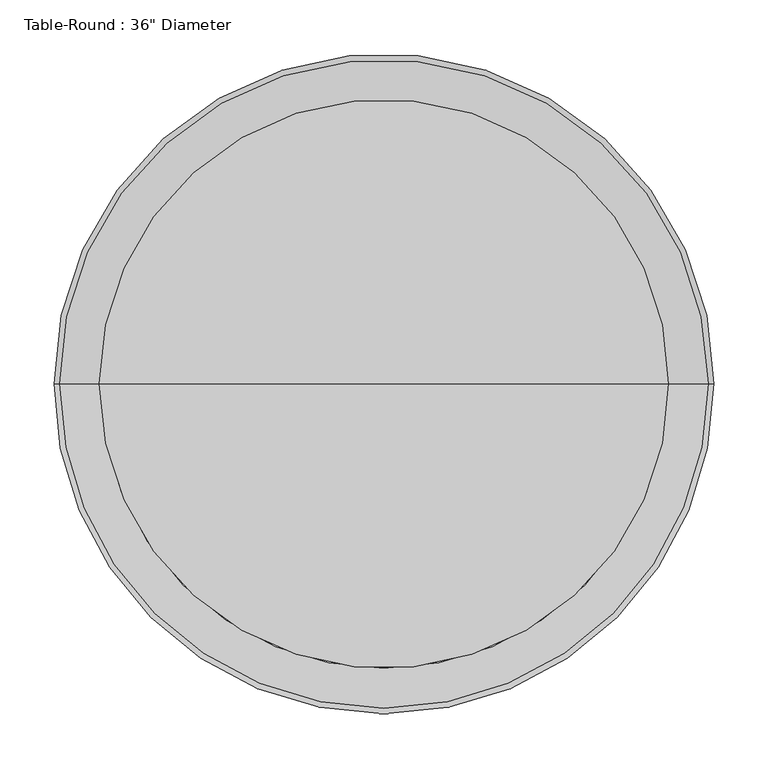
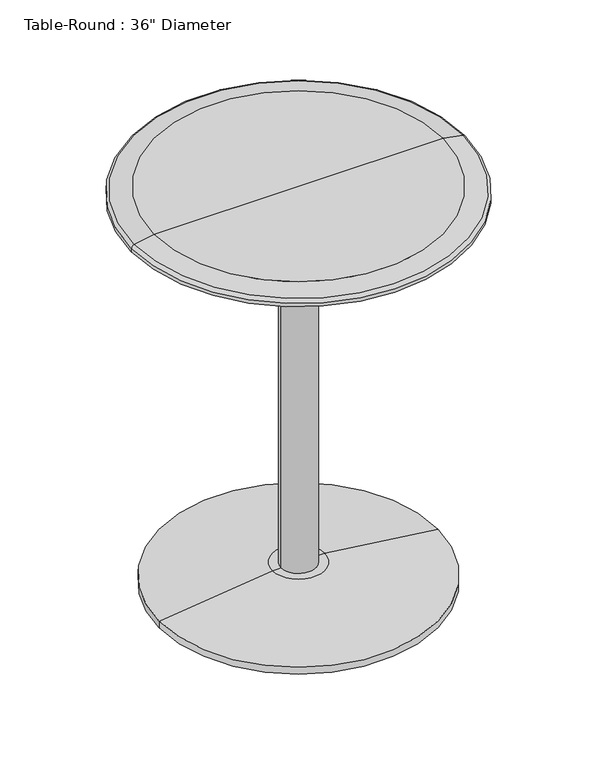
"""IFC4 building model written with IfcOpenShell, lengths in millimetres: furniture geometry."""

from ifc_helpers import new_model, si_unit, point, frame, origin, origin_2d, place, context, project, spatial, polyline, circle_curve, ellipse_curve, trimmed, segment, composite_curve, outline, extrude, source, transform, mapped, element, save
from ifc_brep_helpers import plane_surface, cylinder_surface, revolved_surface, advanced_brep


def furniture_a0cc3393(model_context):
    return source(origin(), model_context, "Body", "SolidModel", [
        extrude(outline(composite_curve([segment(trimmed(circle_curve(origin_2d(), 31.75), [point((-31.75, 0.0))], [point((31.75, 0.0))], False, "CARTESIAN"), True, "CONTINUOUS"), segment(trimmed(circle_curve(origin_2d(), 31.75), [point((31.75, 0.0))], [point((-31.75, 0.0))], False, "CARTESIAN"), True, "CONTINUOUS")], self_intersect=False)), frame((0.0, 0.0, 38.1), z_axis=(0.0, 0.0, 1.0), x_axis=(1.0, 0.0, 0.0)), (0.0, 0.0, 1.0), 704.85),
        advanced_brep(
        [(0.0, 0.0, 742.95), (-304.8, 0.0, 742.95), (304.8, 0.0, 742.95), (262.9011364, 0.0, 762.0), (-262.9011364, 0.0, 762.0), (0.0, 0.0, 762.0), (299.5526659, 0.0, 755.5373465), (-299.5526659, 0.0, 755.5373465), (304.8, 0.0, 749.2838172), (-304.8, 0.0, 749.2838172)],
        [
            (0, 1),
            (1, 2, circle_curve(frame((0.0, 0.0, 742.95), z_axis=(0.0, 0.0, -1.0), x_axis=(-1.0, 0.0, 0.0)), 304.8)),
            (2, 0),
            (2, 1, circle_curve(frame((0.0, 0.0, 742.95), z_axis=(0.0, 0.0, -1.0), x_axis=(-1.0, 0.0, 0.0)), 304.8)),
            (3, 4, circle_curve(frame((0.0, 0.0, 762.0), z_axis=(0.0, 0.0, 1.0), x_axis=(-1.0, 0.0, 0.0)), 262.9011364)),
            (4, 5),
            (5, 3),
            (4, 3, circle_curve(frame((0.0, 0.0, 762.0), z_axis=(0.0, 0.0, 1.0), x_axis=(-1.0, 0.0, 0.0)), 262.9011364)),
            (6, 7, circle_curve(frame((0.0, 0.0, 755.5373465), z_axis=(0.0, 0.0, 1.0), x_axis=(-1.0, 0.0, 0.0)), 299.5526659)),
            (7, 4),
            (3, 6),
            (7, 6, circle_curve(frame((0.0, 0.0, 755.5373465), z_axis=(0.0, 0.0, 1.0), x_axis=(-1.0, 0.0, 0.0)), 299.5526659)),
            (8, 9, circle_curve(frame((0.0, 0.0, 749.2838172), z_axis=(0.0, 0.0, 1.0), x_axis=(-1.0, 0.0, 0.0)), 304.8)),
            (9, 7, circle_curve(frame((-298.45, 0.0, 749.2838172), z_axis=(0.0, 1.0, 0.0), x_axis=(1.0, 0.0, 0.0)), 6.35)),
            (6, 8, circle_curve(frame((298.45, 0.0, 749.2838172), z_axis=(0.0, 1.0, 0.0), x_axis=(-1.0, 0.0, 0.0)), 6.35)),
            (9, 8, circle_curve(frame((0.0, 0.0, 749.2838172), z_axis=(0.0, 0.0, 1.0), x_axis=(-1.0, 0.0, 0.0)), 304.8)),
            (1, 9),
            (8, 2),
        ],
        [
            plane_surface(frame((0.0, 0.0, 742.95), z_axis=(0.0, 0.0, -1.0), x_axis=(-1.0, 0.0, 0.0))),
            plane_surface(frame((0.0, 0.0, 762.0), z_axis=(0.0, 0.0, 1.0), x_axis=(-1.0, 0.0, 0.0))),
            revolved_surface(polyline([(-262.9011364, 0.0, 762.0), (-299.5526659, 0.0, 755.5373465)]), (0.0, 0.0, 838.2), (0.0, 0.0, -1.0)),
            revolved_surface(trimmed(ellipse_curve(frame((-298.45, 0.0, 749.2838172), z_axis=(0.0, -1.0, 0.0), x_axis=(1.0, 0.0, 0.0)), 6.35, 6.35), [point((-299.5526659, 0.0, 755.5373465))], [point((-304.8, 0.0, 749.2838172))], True, "CARTESIAN"), (0.0, 0.0, 838.2), (0.0, 0.0, -1.0)),
            cylinder_surface(frame((0.0, 0.0, 838.2), z_axis=(0.0, 0.0, -1.0), x_axis=(-1.0, 0.0, 0.0)), 304.8),
        ],
        [
            (0, [[1, 2, 3]]),
            (0, [[-3, 4, -1]]),
            (1, [[5, 6, 7]]),
            (1, [[8, -7, -6]]),
            (2, [[9, 10, -5, 11]]),
            (2, [[12, -11, -8, -10]]),
            (3, [[13, 14, -9, 15]]),
            (3, [[16, -15, -12, -14]]),
            (4, [[-2, 17, -13, 18]]),
            (4, [[-4, -18, -16, -17]]),
        ],
    ),
        advanced_brep(
        [(0.0, 0.0, 0.0), (-254.0, 0.0, 0.0), (254.0, 0.0, 0.0), (47.625, 0.0, 38.1), (-47.625, 0.0, 38.1), (0.0, 0.0, 38.1), (254.0, 0.0, 12.7), (-254.0, 0.0, 12.7)],
        [
            (0, 1),
            (1, 2, circle_curve(frame((0.0, 0.0, 0.0), z_axis=(0.0, 0.0, -1.0), x_axis=(-1.0, 0.0, 0.0)), 254.0)),
            (2, 0),
            (2, 1, circle_curve(frame((0.0, 0.0, 0.0), z_axis=(0.0, 0.0, -1.0), x_axis=(-1.0, 0.0, 0.0)), 254.0)),
            (3, 4, circle_curve(frame((0.0, 0.0, 38.1), z_axis=(0.0, 0.0, 1.0), x_axis=(-1.0, 0.0, 0.0)), 47.625)),
            (4, 5),
            (5, 3),
            (4, 3, circle_curve(frame((0.0, 0.0, 38.1), z_axis=(0.0, 0.0, 1.0), x_axis=(-1.0, 0.0, 0.0)), 47.625)),
            (6, 7, circle_curve(frame((0.0, 0.0, 12.7), z_axis=(0.0, 0.0, 1.0), x_axis=(-1.0, 0.0, 0.0)), 254.0)),
            (7, 4),
            (3, 6),
            (7, 6, circle_curve(frame((0.0, 0.0, 12.7), z_axis=(0.0, 0.0, 1.0), x_axis=(-1.0, 0.0, 0.0)), 254.0)),
            (1, 7),
            (6, 2),
        ],
        [
            plane_surface(frame((0.0, 0.0, 0.0), z_axis=(0.0, 0.0, -1.0), x_axis=(-1.0, 0.0, 0.0))),
            plane_surface(frame((0.0, 0.0, 38.1), z_axis=(0.0, 0.0, 1.0), x_axis=(-1.0, 0.0, 0.0))),
            revolved_surface(polyline([(-47.625, 0.0, 38.1), (-254.0, 0.0, 12.7)]), (0.0, 0.0, 215.9), (0.0, 0.0, -1.0)),
            cylinder_surface(frame((0.0, 0.0, 215.9), z_axis=(0.0, 0.0, -1.0), x_axis=(-1.0, 0.0, 0.0)), 254.0),
        ],
        [
            (0, [[1, 2, 3]]),
            (0, [[-3, 4, -1]]),
            (1, [[5, 6, 7]]),
            (1, [[8, -7, -6]]),
            (2, [[9, 10, -5, 11]]),
            (2, [[12, -11, -8, -10]]),
            (3, [[-2, 13, -9, 14]]),
            (3, [[-4, -14, -12, -13]]),
        ],
    ),
    ])


if __name__ == "__main__":
    model = new_model("IFC4")
    model_context = context("Model", 3, world=origin())
    ifc_project = project(units=[si_unit("LENGTHUNIT", "METRE", prefix="MILLI")], contexts=[model_context])
    site = spatial("IfcSite", under=ifc_project)
    building = spatial("IfcBuilding", under=site)
    placement = place(None, origin())
    furniture_shape = furniture_a0cc3393(model_context)
    element("IfcFurniture", 1, ObjectType="Table-Round : 36\" Diameter", at=placement, inside=building, context=model_context, shape_type="MappedRepresentation", body=[
        mapped(furniture_shape, transform((0.0, 0.0, 0.0), x_axis=(1.0, 0.0, 0.0), y_axis=(0.0, 1.0, 0.0), z_axis=(0.0, 0.0, 1.0))),
    ])
    save(model, "model.ifc")

# Revit data of these elements
# Type "Table-Round : 36\" Diameter"
#   Assembly Code = "E2020200"
#   Base Radius = 0' - 10"
#   Height = 2' - 6"
#   Radius = 1' - 0"
#   Base Material = Steel, Chrome Plated
#   Top Material = Birch
#   Default Elevation = 0
# Element 1 (IfcFurniture, "Table-Round : 36\" Diameter")
#   Materials on its faces: "Steel, Chrome Plated", "Birch"
# Materials
#   "Steel, Chrome Plated": class "Metal", colour RGB 17 17 17, transparency 0, Description = "Chromiuim plated steel", Cost = 0
#   "Birch": class "Wood", colour RGB 224 178 126, transparency 0, Description = "Betula Alleghaniensis", Cost = 0
